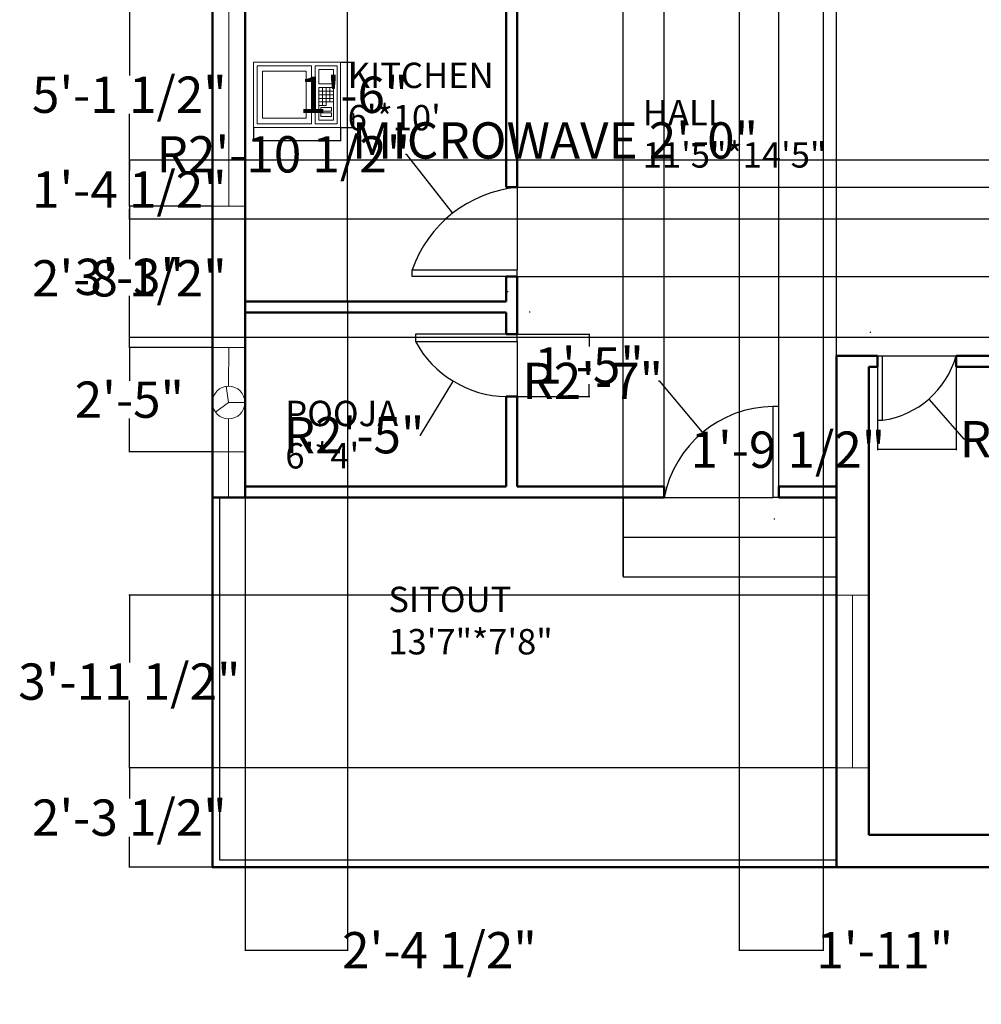
# Model space of a CAD drawing. Units: inches. Extents: x 430 to 924, y 262 to 758.
# Tile 1 of 3: x 430 to 695, y 262 to 534. Entities that reach past the tile are written whole.
import ezdxf

# ---------------------------------------------------------------- set-up
doc = ezdxf.new("R2010")
doc.units = ezdxf.units.IN
doc.header["$MEASUREMENT"] = 0
for name, color, linetype, lineweight in [('A-ANNO-DIMS', 2, 'Continuous', 18), ('A-AREA-IDEN', 7, 'Continuous', 25), ('A-DOOR', 4, 'Continuous', 25), ('A-EQPM', 8, 'Continuous', 18), ('A-FLOR', 7, 'Continuous', 25), ('A-FLOR-CASE', 9, 'Continuous', 25), ('A-FLOR-STRS', 7, 'Continuous', 25), ('A-GLAZ', 3, 'Continuous', 18), ('A-WALL', 7, 'Continuous', 50), ('M-HVAC-EQPM', 4, 'Continuous', 18)]:
    doc.layers.add(name, color=color, linetype=linetype, lineweight=lineweight)
doc.styles.get("Standard").update_dxf_attribs({"font": 'arial.ttf'})
doc.dimstyles.get("Standard").update_dxf_attribs({"dimtxt": 10, "dimasz": 0.18, "dimexe": 0.18, "dimexo": 0.0625, "dimgap": 0.09, "dimtad": 0, "dimtih": 1, "dimtoh": 1, "dimdec": 0, "dimzin": 0, "dimdsep": 46, "dimlunit": 3, "dimtxsty": 'Standard', "dimcen": 0.09, "dimadec": 0, "dimazin": 0, "dimtfac": 1, "dimtdec": 0, "dimtofl": 0, "dimtmove": 0, "dimatfit": 3, "dimfxl": 1, "dimtolj": 1, "dimtzin": 0, "dimarcsym": 0})

# ---------------------------------------------------------------- blocks, each defined once
blk = doc.blocks.new('Microwave')
for p, q in [((19, 7), (19, 11)), ((20, 11), (20, 7)), ((21, 7), (21, 11)), ((18, 10), (22, 10)), ((22, 9), (18, 9)), ((18, 8), (22, 8)), ((22, 7), (18, 7)), ((20, 6), (18, 6)), ((19, 6), (19, 7)), ((20, 7), (20, 6))]:
    blk.add_line(p, q)
for points in [[(0, 0), (0, 18), (24, 18), (24, 0)], [(1, 1), (1, 17), (16, 17), (16, 1)], [(17, 1), (17, 17), (23, 17), (23, 1)], [(2.5, 2.5), (2.5, 15.5), (14.5, 15.5), (14.5, 2.5)], [(18, 12), (18, 16), (22, 16), (22, 12)], [(18, 2), (18, 11), (22, 11), (22, 2)], [(18.5, 4.5), (18.5, 5.5), (21.5, 5.5), (21.5, 4.5)], [(18.5, 3), (18.5, 4), (21.5, 4), (21.5, 3)]]:
    blk.add_lwpolyline(points, close=True)
blk = doc.blocks.new('*D9')
at = {"layer": 'A-ANNO-DIMS', "color": 0, "lineweight": -2, "transparency": 16777216}
for p, q in [((494.67, 503.98), (494.67, 500.27)), ((518.67, 503.98), (518.67, 500.27)), ((494.85, 500.45), (518.49, 500.45)), ((518.67, 500.45), (518.85, 500.45))]:
    blk.add_line(p, q, dxfattribs=at)
at = {"layer": 'A-ANNO-DIMS', "color": 0, "transparency": 16777216}
for points in [[(494.85, 500.48), (494.85, 500.42), (494.67, 500.45)], [(518.49, 500.48), (518.49, 500.42), (518.67, 500.45)]]:
    blk.add_solid(points, dxfattribs=at)
at = {"layer": 'Defpoints', "color": 0, "transparency": 16777216}
for p in [(494.67, 504.05), (518.67, 504.05), (518.67, 500.45)]:
    blk.add_point(p, dxfattribs=at)
at = {"layer": 'A-ANNO-DIMS', "color": 0, "transparency": 16777216, "insert": (577.79, 500.45), "char_height": 10, "attachment_point": 5}
blk.add_mtext('\\A1;MICROWAVE 2\'-0"', dxfattribs=at)
blk = doc.blocks.new('*D10')
at = {"layer": 'A-ANNO-DIMS', "color": 0, "lineweight": -2, "transparency": 16777216}
for p, q in [((518.73, 522.05), (522.45, 522.05)), ((522.27, 521.87), (522.27, 518.24)), ((522.27, 504.23), (522.27, 507.85)), ((518.73, 504.05), (522.45, 504.05))]:
    blk.add_line(p, q, dxfattribs=at)
at = {"layer": 'A-ANNO-DIMS', "color": 0, "transparency": 16777216}
for points in [[(522.24, 521.87), (522.3, 521.87), (522.27, 522.05)], [(522.24, 504.23), (522.3, 504.23), (522.27, 504.05)]]:
    blk.add_solid(points, dxfattribs=at)
at = {"layer": 'Defpoints', "color": 0, "transparency": 16777216}
for p in [(518.67, 522.05), (522.27, 522.05), (518.67, 504.05)]:
    blk.add_point(p, dxfattribs=at)
at = {"layer": 'A-ANNO-DIMS', "color": 0, "transparency": 16777216, "insert": (522.27, 513.05), "char_height": 10, "attachment_point": 5}
blk.add_mtext('\\A1;1\'-6"', dxfattribs=at)
blk = doc.blocks.new('*D11')
at = {"layer": 'A-ANNO-DIMS', "color": 0, "lineweight": -2, "transparency": 16777216}
for p, q in [((523.75, 547.42), (523.75, 542.8)), ((553.75, 547.42), (553.75, 542.8)), ((523.93, 542.98), (553.57, 542.98)), ((553.75, 542.98), (553.93, 542.98))]:
    blk.add_line(p, q, dxfattribs=at)
at = {"layer": 'A-ANNO-DIMS', "color": 0, "transparency": 16777216}
for points in [[(523.93, 543.01), (523.93, 542.95), (523.75, 542.98)], [(553.57, 543.01), (553.57, 542.95), (553.75, 542.98)]]:
    blk.add_solid(points, dxfattribs=at)
at = {"layer": 'Defpoints', "color": 0, "transparency": 16777216}
for p in [(523.75, 547.48), (553.75, 547.48), (553.75, 542.98)]:
    blk.add_point(p, dxfattribs=at)
at = {"layer": 'A-ANNO-DIMS', "color": 0, "transparency": 16777216, "insert": (585.53, 542.98), "char_height": 10, "attachment_point": 5}
blk.add_mtext('\\A1;SINK 2\'-6"', dxfattribs=at)
blk = doc.blocks.new('*D28')
at = {"layer": 'A-ANNO-DIMS', "color": 0, "lineweight": -2, "transparency": 16777216}
for p, q in [((483.25, 543.78), (460.24, 543.78)), ((460.42, 543.6), (460.42, 518.31)), ((460.42, 482.49), (460.42, 507.78)), ((483.25, 482.31), (460.24, 482.31))]:
    blk.add_line(p, q, dxfattribs=at)
at = {"layer": 'A-ANNO-DIMS', "color": 0, "transparency": 16777216}
for points in [[(460.39, 543.6), (460.45, 543.6), (460.42, 543.78)], [(460.39, 482.49), (460.45, 482.49), (460.42, 482.31)]]:
    blk.add_solid(points, dxfattribs=at)
at = {"layer": 'Defpoints', "color": 0, "transparency": 16777216}
for p in [(483.32, 543.78), (460.42, 482.31), (483.32, 482.31)]:
    blk.add_point(p, dxfattribs=at)
at = {"layer": 'A-ANNO-DIMS', "color": 0, "transparency": 16777216, "insert": (460.42, 513.05), "char_height": 10, "attachment_point": 5}
blk.add_mtext('\\A1;5\'-1 1/2"', dxfattribs=at)
blk = doc.blocks.new('*D29')
at = {"layer": 'A-ANNO-DIMS', "color": 0, "lineweight": -2, "transparency": 16777216}
for p, q in [((483.25, 482.31), (460.24, 482.31)), ((460.42, 482.13), (460.42, 468.03)), ((460.42, 443.54), (460.42, 457.64)), ((483.25, 443.36), (460.24, 443.36))]:
    blk.add_line(p, q, dxfattribs=at)
at = {"layer": 'A-ANNO-DIMS', "color": 0, "transparency": 16777216}
for points in [[(460.39, 482.13), (460.45, 482.13), (460.42, 482.31)], [(460.39, 443.54), (460.45, 443.54), (460.42, 443.36)]]:
    blk.add_solid(points, dxfattribs=at)
at = {"layer": 'Defpoints', "color": 0, "transparency": 16777216}
for p in [(483.32, 482.31), (460.42, 443.36), (483.32, 443.36)]:
    blk.add_point(p, dxfattribs=at)
at = {"layer": 'A-ANNO-DIMS', "color": 0, "transparency": 16777216, "insert": (460.42, 462.84), "char_height": 10, "attachment_point": 5}
blk.add_mtext('\\A1;3\'-3"', dxfattribs=at)
blk = doc.blocks.new('*D30')
at = {"layer": 'A-ANNO-DIMS', "color": 0, "lineweight": -2, "transparency": 16777216}
for p, q in [((483.25, 443.36), (460.24, 443.36)), ((460.42, 443.18), (460.42, 434.17)), ((460.42, 414.78), (460.42, 423.78)), ((483.25, 414.6), (460.24, 414.6))]:
    blk.add_line(p, q, dxfattribs=at)
at = {"layer": 'A-ANNO-DIMS', "color": 0, "transparency": 16777216}
for points in [[(460.39, 443.18), (460.45, 443.18), (460.42, 443.36)], [(460.39, 414.78), (460.45, 414.78), (460.42, 414.6)]]:
    blk.add_solid(points, dxfattribs=at)
at = {"layer": 'Defpoints', "color": 0, "transparency": 16777216}
for p in [(483.32, 443.36), (460.42, 414.6), (483.32, 414.6)]:
    blk.add_point(p, dxfattribs=at)
at = {"layer": 'A-ANNO-DIMS', "color": 0, "transparency": 16777216, "insert": (460.42, 428.98), "char_height": 10, "attachment_point": 5}
blk.add_mtext('\\A1;2\'-5"', dxfattribs=at)
blk = doc.blocks.new('*D33')
at = {"layer": 'A-ANNO-DIMS', "color": 0, "lineweight": -2, "transparency": 16777216}
for p, q in [((655.25, 327.47), (460.24, 327.47)), ((460.42, 327.29), (460.42, 319.03)), ((460.42, 300.23), (460.42, 308.5)), ((655.25, 300.05), (460.24, 300.05))]:
    blk.add_line(p, q, dxfattribs=at)
at = {"layer": 'A-ANNO-DIMS', "color": 0, "transparency": 16777216}
for points in [[(460.39, 327.29), (460.45, 327.29), (460.42, 327.47)], [(460.39, 300.23), (460.45, 300.23), (460.42, 300.05)]]:
    blk.add_solid(points, dxfattribs=at)
at = {"layer": 'Defpoints', "color": 0, "transparency": 16777216}
for p in [(460.42, 327.47), (655.32, 327.47), (655.32, 300.05)]:
    blk.add_point(p, dxfattribs=at)
at = {"layer": 'A-ANNO-DIMS', "color": 0, "transparency": 16777216, "insert": (460.42, 313.76), "char_height": 10, "attachment_point": 5}
blk.add_mtext('\\A1;2\'-3 1/2"', dxfattribs=at)
blk = doc.blocks.new('*D34')
at = {"layer": 'A-ANNO-DIMS', "color": 0, "lineweight": -2, "transparency": 16777216}
for p, q in [((655.25, 375.05), (460.24, 375.05)), ((460.42, 374.87), (460.42, 356.53)), ((460.42, 327.65), (460.42, 346)), ((655.25, 327.47), (460.24, 327.47))]:
    blk.add_line(p, q, dxfattribs=at)
at = {"layer": 'A-ANNO-DIMS', "color": 0, "transparency": 16777216}
for points in [[(460.39, 374.87), (460.45, 374.87), (460.42, 375.05)], [(460.39, 327.65), (460.45, 327.65), (460.42, 327.47)]]:
    blk.add_solid(points, dxfattribs=at)
at = {"layer": 'Defpoints', "color": 0, "transparency": 16777216}
for p in [(460.42, 375.05), (655.32, 375.05), (655.32, 327.47)]:
    blk.add_point(p, dxfattribs=at)
at = {"layer": 'A-ANNO-DIMS', "color": 0, "transparency": 16777216, "insert": (460.42, 351.26), "char_height": 10, "attachment_point": 5}
blk.add_mtext('\\A1;3\'-11 1/2"', dxfattribs=at)
blk = doc.blocks.new('*D35')
at = {"layer": 'A-ANNO-DIMS', "color": 0, "lineweight": -2, "transparency": 16777216}
for p, q in [((596.53, 380.21), (596.53, 743.09)), ((596.71, 742.91), (608.45, 742.91)), ((655.14, 742.91), (643.39, 742.91)), ((655.32, 380.21), (655.32, 743.09))]:
    blk.add_line(p, q, dxfattribs=at)
at = {"layer": 'A-ANNO-DIMS', "color": 0, "transparency": 16777216}
for points in [[(596.71, 742.94), (596.71, 742.88), (596.53, 742.91)], [(655.14, 742.94), (655.14, 742.88), (655.32, 742.91)]]:
    blk.add_solid(points, dxfattribs=at)
at = {"layer": 'Defpoints', "color": 0, "transparency": 16777216}
for p in [(655.32, 742.91), (596.53, 380.15), (655.32, 380.15)]:
    blk.add_point(p, dxfattribs=at)
at = {"layer": 'A-ANNO-DIMS', "color": 0, "transparency": 16777216, "insert": (625.92, 742.91), "char_height": 10, "attachment_point": 5}
blk.add_mtext('\\A1;4\'-11"', dxfattribs=at)
blk = doc.blocks.new('*D39')
at = {"layer": 'A-ANNO-DIMS', "color": 0, "lineweight": -2, "transparency": 16777216}
for p, q in [((752.25, 478.73), (460.24, 478.73)), ((460.42, 478.55), (460.42, 467.71)), ((460.42, 446.34), (460.42, 457.18)), ((752.25, 446.16), (460.24, 446.16))]:
    blk.add_line(p, q, dxfattribs=at)
at = {"layer": 'A-ANNO-DIMS', "color": 0, "transparency": 16777216}
for points in [[(460.39, 478.55), (460.45, 478.55), (460.42, 478.73)], [(460.39, 446.34), (460.45, 446.34), (460.42, 446.16)]]:
    blk.add_solid(points, dxfattribs=at)
at = {"layer": 'Defpoints', "color": 0, "transparency": 16777216}
for p in [(460.42, 478.73), (752.32, 478.73), (752.32, 446.16)]:
    blk.add_point(p, dxfattribs=at)
at = {"layer": 'A-ANNO-DIMS', "color": 0, "transparency": 16777216, "insert": (460.42, 462.44), "char_height": 10, "attachment_point": 5}
blk.add_mtext('\\A1;2\'-8 1/2"', dxfattribs=at)
blk = doc.blocks.new('*D40')
at = {"layer": 'A-ANNO-DIMS', "color": 0, "lineweight": -2, "transparency": 16777216}
for p, q in [((752.25, 495.05), (460.24, 495.05)), ((460.42, 494.87), (460.42, 492.15)), ((460.42, 478.91), (460.42, 481.63)), ((752.25, 478.73), (460.24, 478.73))]:
    blk.add_line(p, q, dxfattribs=at)
at = {"layer": 'A-ANNO-DIMS', "color": 0, "transparency": 16777216}
for points in [[(460.39, 494.87), (460.45, 494.87), (460.42, 495.05)], [(460.39, 478.91), (460.45, 478.91), (460.42, 478.73)]]:
    blk.add_solid(points, dxfattribs=at)
at = {"layer": 'Defpoints', "color": 0, "transparency": 16777216}
for p in [(460.42, 495.05), (752.32, 495.05), (752.32, 478.73)]:
    blk.add_point(p, dxfattribs=at)
at = {"layer": 'A-ANNO-DIMS', "color": 0, "transparency": 16777216, "insert": (460.42, 486.89), "char_height": 10, "attachment_point": 5}
blk.add_mtext('\\A1;1\'-4 1/2"', dxfattribs=at)
blk = doc.blocks.new('*D42')
at = {"layer": 'A-ANNO-DIMS', "color": 0, "lineweight": -2, "transparency": 16777216}
for p, q in [((492.32, 455.99), (492.32, 277.02)), ((520.6, 455.99), (520.6, 277.02)), ((492.5, 277.2), (520.42, 277.2)), ((520.6, 277.2), (520.78, 277.2))]:
    blk.add_line(p, q, dxfattribs=at)
at = {"layer": 'A-ANNO-DIMS', "color": 0, "transparency": 16777216}
for points in [[(492.5, 277.23), (492.5, 277.17), (492.32, 277.2)], [(520.42, 277.23), (520.42, 277.17), (520.6, 277.2)]]:
    blk.add_solid(points, dxfattribs=at)
at = {"layer": 'Defpoints', "color": 0, "transparency": 16777216}
for p in [(492.32, 456.05), (520.6, 456.05), (520.6, 277.2)]:
    blk.add_point(p, dxfattribs=at)
at = {"layer": 'A-ANNO-DIMS', "color": 0, "transparency": 16777216, "insert": (545.9, 277.2), "char_height": 10, "attachment_point": 5}
blk.add_mtext('\\A1;2\'-4 1/2"', dxfattribs=at)
blk = doc.blocks.new('*D44')
at = {"layer": 'A-ANNO-DIMS', "color": 0, "lineweight": -2, "transparency": 16777216}
for p, q in [((567.38, 487.53), (854.35, 487.53)), ((854.17, 487.35), (854.17, 480.5)), ((854.17, 463.13), (854.17, 469.98)), ((567.38, 462.95), (854.35, 462.95))]:
    blk.add_line(p, q, dxfattribs=at)
at = {"layer": 'A-ANNO-DIMS', "color": 0, "transparency": 16777216}
for points in [[(854.14, 487.35), (854.2, 487.35), (854.17, 487.53)], [(854.14, 463.13), (854.2, 463.13), (854.17, 462.95)]]:
    blk.add_solid(points, dxfattribs=at)
at = {"layer": 'Defpoints', "color": 0, "transparency": 16777216}
for p in [(567.32, 487.53), (854.17, 487.53), (567.32, 462.95)]:
    blk.add_point(p, dxfattribs=at)
at = {"layer": 'A-ANNO-DIMS', "color": 0, "transparency": 16777216, "insert": (854.17, 475.24), "char_height": 10, "attachment_point": 5}
blk.add_mtext('\\A1;2\'-0 1/2"', dxfattribs=at)
blk = doc.blocks.new('*D46')
at = {"layer": 'A-ANNO-DIMS', "color": 0, "lineweight": -2, "transparency": 16777216}
for p, q in [((628.55, 575.99), (628.55, 277.02)), ((651.7, 575.99), (651.7, 277.02)), ((628.73, 277.2), (651.52, 277.2)), ((651.7, 277.2), (651.88, 277.2))]:
    blk.add_line(p, q, dxfattribs=at)
at = {"layer": 'A-ANNO-DIMS', "color": 0, "transparency": 16777216}
for points in [[(628.73, 277.23), (628.73, 277.17), (628.55, 277.2)], [(651.52, 277.23), (651.52, 277.17), (651.7, 277.2)]]:
    blk.add_solid(points, dxfattribs=at)
at = {"layer": 'Defpoints', "color": 0, "transparency": 16777216}
for p in [(628.55, 576.05), (651.7, 576.05), (651.7, 277.2)]:
    blk.add_point(p, dxfattribs=at)
at = {"layer": 'A-ANNO-DIMS', "color": 0, "transparency": 16777216, "insert": (668.68, 277.2), "char_height": 10, "attachment_point": 5}
blk.add_mtext('\\A1;1\'-11"', dxfattribs=at)
blk = doc.blocks.new('*D48')
at = {"layer": 'A-ANNO-DIMS', "color": 0, "lineweight": -2, "transparency": 16777216}
for p, q in [((607.88, 405.12), (607.88, 743.09)), ((608.06, 742.91), (639.32, 742.91)), ((639.5, 405.12), (639.5, 743.09)), ((639.5, 742.91), (639.68, 742.91))]:
    blk.add_line(p, q, dxfattribs=at)
at = {"layer": 'A-ANNO-DIMS', "color": 0, "transparency": 16777216}
for points in [[(608.06, 742.94), (608.06, 742.88), (607.88, 742.91)], [(639.32, 742.94), (639.32, 742.88), (639.5, 742.91)]]:
    blk.add_solid(points, dxfattribs=at)
at = {"layer": 'Defpoints', "color": 0, "transparency": 16777216}
for p in [(639.5, 742.91), (607.88, 405.05), (639.5, 405.05)]:
    blk.add_point(p, dxfattribs=at)
at = {"layer": 'A-ANNO-DIMS', "color": 0, "transparency": 16777216, "insert": (664.79, 742.91), "char_height": 10, "attachment_point": 5}
blk.add_mtext('\\A1;2\'-7 1/2"', dxfattribs=at)
blk = doc.blocks.new('*D49')
at = {"layer": 'A-ANNO-DIMS', "color": 0, "lineweight": -2, "transparency": 16777216}
for p, q in [((666.71, 437.99), (666.71, 415.02)), ((688.33, 437.99), (688.33, 415.02)), ((666.71, 415.2), (666.53, 415.2)), ((688.15, 415.2), (666.89, 415.2))]:
    blk.add_line(p, q, dxfattribs=at)
at = {"layer": 'A-ANNO-DIMS', "color": 0, "transparency": 16777216}
for points in [[(666.89, 415.23), (666.89, 415.17), (666.71, 415.2)], [(688.15, 415.23), (688.15, 415.17), (688.33, 415.2)]]:
    blk.add_solid(points, dxfattribs=at)
at = {"layer": 'Defpoints', "color": 0, "transparency": 16777216}
for p in [(666.71, 438.05), (688.33, 438.05), (666.71, 415.2)]:
    blk.add_point(p, dxfattribs=at)
at = {"layer": 'A-ANNO-DIMS', "color": 0, "transparency": 16777216, "insert": (641.97, 415.2), "char_height": 10, "attachment_point": 5}
blk.add_mtext('\\A1;1\'-9 1/2"', dxfattribs=at)
blk = doc.blocks.new('*D50')
at = {"layer": 'A-ANNO-DIMS', "color": 0, "lineweight": -2, "transparency": 16777216}
for p, q in [((564.38, 447.02), (587.35, 447.02)), ((587.17, 446.84), (587.17, 443.63)), ((587.17, 430.02), (587.17, 433.23)), ((564.38, 429.84), (587.35, 429.84))]:
    blk.add_line(p, q, dxfattribs=at)
at = {"layer": 'A-ANNO-DIMS', "color": 0, "transparency": 16777216}
for points in [[(587.14, 446.84), (587.2, 446.84), (587.17, 447.02)], [(587.14, 430.02), (587.2, 430.02), (587.17, 429.84)]]:
    blk.add_solid(points, dxfattribs=at)
at = {"layer": 'Defpoints', "color": 0, "transparency": 16777216}
for p in [(564.32, 447.02), (564.32, 429.84), (587.17, 429.84)]:
    blk.add_point(p, dxfattribs=at)
at = {"layer": 'A-ANNO-DIMS', "color": 0, "transparency": 16777216, "insert": (587.17, 438.43), "char_height": 10, "attachment_point": 5}
blk.add_mtext('\\A1;1\'-5"', dxfattribs=at)
blk = doc.blocks.new('*D54')
at = {"layer": 'A-ANNO-DIMS', "color": 0, "lineweight": -2, "transparency": 16777216}
for p, q in [((536.58, 496.62), (536.76, 496.62)), ((536.76, 496.62), (549.43, 480.49)), ((570.75, 453.23), (570.93, 453.23)), ((570.84, 453.14), (570.84, 453.32))]:
    blk.add_line(p, q, dxfattribs=at)
at = {"layer": 'A-ANNO-DIMS', "color": 0, "transparency": 16777216}
blk.add_solid([(549.45, 480.51), (549.4, 480.47), (549.54, 480.35)], dxfattribs=at)
at = {"layer": 'Defpoints', "color": 0, "transparency": 16777216}
for p in [(549.54, 480.35), (570.84, 453.23)]:
    blk.add_point(p, dxfattribs=at)
at = {"layer": 'A-ANNO-DIMS', "color": 0, "transparency": 16777216, "insert": (502.88, 496.62), "char_height": 10, "attachment_point": 5}
blk.add_mtext('\\A1;R2\'-10 1/2"', dxfattribs=at)
blk = doc.blocks.new('*D55')
at = {"layer": 'A-ANNO-DIMS', "color": 0, "lineweight": -2, "transparency": 16777216}
for p, q in [((564.69, 458.82), (564.87, 458.82)), ((564.78, 458.73), (564.78, 458.91)), ((540.71, 419.18), (549.64, 433.89)), ((540.53, 419.18), (540.71, 419.18))]:
    blk.add_line(p, q, dxfattribs=at)
at = {"layer": 'A-ANNO-DIMS', "color": 0, "transparency": 16777216}
blk.add_solid([(549.61, 433.91), (549.67, 433.87), (549.73, 434.04)], dxfattribs=at)
at = {"layer": 'Defpoints', "color": 0, "transparency": 16777216}
for p in [(564.78, 458.82), (549.73, 434.04)]:
    blk.add_point(p, dxfattribs=at)
at = {"layer": 'A-ANNO-DIMS', "color": 0, "transparency": 16777216, "insert": (522.36, 419.18), "char_height": 10, "attachment_point": 5}
blk.add_mtext('\\A1;R2\'-5"', dxfattribs=at)
blk = doc.blocks.new('*D56')
at = {"layer": 'A-ANNO-DIMS', "color": 0, "lineweight": -2, "transparency": 16777216}
for p, q in [((606.31, 434.15), (606.49, 434.15)), ((606.49, 434.15), (618.29, 420.04)), ((638.18, 396.15), (638.36, 396.15)), ((638.27, 396.06), (638.27, 396.24))]:
    blk.add_line(p, q, dxfattribs=at)
at = {"layer": 'A-ANNO-DIMS', "color": 0, "transparency": 16777216}
blk.add_solid([(618.32, 420.06), (618.27, 420.02), (618.41, 419.9)], dxfattribs=at)
at = {"layer": 'Defpoints', "color": 0, "transparency": 16777216}
for p in [(618.41, 419.9), (638.27, 396.15)]:
    blk.add_point(p, dxfattribs=at)
at = {"layer": 'A-ANNO-DIMS', "color": 0, "transparency": 16777216, "insert": (588.15, 434.15), "char_height": 10, "attachment_point": 5}
blk.add_mtext('\\A1;R2\'-7"', dxfattribs=at)
blk = doc.blocks.new('*D57')
at = {"layer": 'A-ANNO-DIMS', "color": 0, "lineweight": -2, "transparency": 16777216}
for p, q in [((664.61, 447.63), (664.79, 447.63)), ((664.7, 447.54), (664.7, 447.72)), ((690.53, 418.08), (680.96, 429.02)), ((690.71, 418.08), (690.53, 418.08))]:
    blk.add_line(p, q, dxfattribs=at)
at = {"layer": 'A-ANNO-DIMS', "color": 0, "transparency": 16777216}
blk.add_solid([(680.98, 429.04), (680.94, 429), (680.84, 429.16)], dxfattribs=at)
at = {"layer": 'Defpoints', "color": 0, "transparency": 16777216}
for p in [(664.7, 447.63), (680.84, 429.16)]:
    blk.add_point(p, dxfattribs=at)
at = {"layer": 'A-ANNO-DIMS', "color": 0, "transparency": 16777216, "insert": (720.53, 418.08), "char_height": 10, "attachment_point": 5}
blk.add_mtext('\\A1;R2\'-0 1/2"', dxfattribs=at)

msp = doc.modelspace()

# ---------------------------------------------------------------- linework, layer by layer
at = {"layer": 'A-DOOR'}
for p, q in [((567.32, 487.53), (567.32, 464.78)), ((538.34, 462.95), (538.34, 464.78)), ((538.34, 464.78), (567.32, 464.78)), ((567.32, 462.95), (567.32, 464.78)), ((564.32, 462.95), (538.34, 462.95)), ((567.32, 447.02), (539.28, 447.02)), ((539.28, 447.02), (539.28, 445.04)), ((567.32, 445.04), (567.32, 447.02)), ((539.28, 445.04), (567.32, 445.04)), ((567.32, 445.04), (567.32, 429.84)), ((666.71, 441.05), (688.33, 441.05)), ((668.05, 423.33), (668.05, 441.05)), ((666.71, 438.05), (666.71, 423.33)), ((639.5, 427.11), (637.84, 427.11)), ((637.84, 427.11), (637.84, 402.14)), ((639.5, 405.05), (639.5, 427.11)), ((666.71, 423.33), (668.05, 423.33)), ((607.88, 402.05), (637.84, 402.05)), ((637.84, 402.14), (639.5, 402.14))]:
    msp.add_line(p, q, dxfattribs=at)
for centre, radius, start, end in [((570.84, 453.23), 34.49, 95.8576, 160.4254), ((564.78, 458.82), 28.98, 208.3786, 269.0869), ((664.7, 447.63), 24.53, 277.8641, 344.4616), ((638.27, 396.15), 30.96, 90.8013, 169.0102)]:
    msp.add_arc(centre, radius, start, end, dxfattribs=at)
at = {"layer": 'A-FLOR'}
msp.add_lwpolyline([(655.32, 302.05), (485.32, 302.05), (485.32, 402.05)], dxfattribs=at)
at = {"layer": 'A-FLOR-CASE'}
msp.add_line((520.6, 456.05), (520.6, 541.01), dxfattribs=at)
at = {"layer": 'A-FLOR-STRS'}
for p, q in [((596.53, 402.05), (596.53, 380.15)), ((596.53, 391.1), (655.32, 391.1)), ((596.53, 380.15), (655.32, 380.15))]:
    msp.add_line(p, q, dxfattribs=at)
at = {"layer": 'A-GLAZ'}
for p, q in [((487.82, 543.78), (487.82, 482.31)), ((483.32, 482.31), (492.32, 482.31)), ((487.82, 443.36), (487.77, 432.71)), ((487.77, 423.71), (487.77, 402.05)), ((483.32, 414.6), (492.32, 414.6)), ((655.32, 375.05), (664.32, 375.05)), ((659.82, 375.05), (659.82, 327.47)), ((655.32, 327.47), (664.32, 327.47))]:
    msp.add_line(p, q, dxfattribs=at)
msp.add_lwpolyline([(483.32, 443.36), (492.32, 443.36)], dxfattribs=at)
at = {"layer": 'A-WALL'}
for p, q in [((492.32, 402.05), (492.32, 576.05)), ((564.32, 498.05), (564.32, 576.05)), ((567.32, 498.05), (567.32, 576.05)), ((564.32, 498.05), (564.32, 487.53)), ((567.32, 487.53), (567.32, 498.05)), ((564.32, 487.53), (567.32, 487.53)), ((564.32, 462.95), (567.32, 462.95)), ((564.32, 456.05), (564.32, 462.95)), ((567.32, 447.02), (567.32, 462.95)), ((492.32, 456.05), (564.32, 456.05)), ((492.32, 453.05), (564.32, 453.05)), ((564.32, 447.02), (564.32, 453.05)), ((564.32, 447.02), (567.32, 447.02)), ((655.32, 309.05), (655.32, 441.05)), ((664.32, 441.05), (655.32, 441.05)), ((666.71, 441.05), (664.32, 441.05)), ((666.71, 441.05), (666.71, 438.05)), ((706.32, 441.05), (688.33, 441.05)), ((688.33, 441.05), (688.33, 438.05)), ((664.32, 309.05), (664.32, 438.05)), ((666.71, 438.05), (664.32, 438.05)), ((703.32, 438.05), (688.33, 438.05)), ((564.32, 405.05), (564.32, 429.84)), ((564.32, 429.84), (567.32, 429.84)), ((567.32, 405.05), (567.32, 429.84)), ((492.32, 405.05), (564.32, 405.05)), ((567.32, 405.05), (607.88, 405.05)), ((607.88, 405.05), (607.88, 402.05)), ((655.32, 405.05), (639.5, 405.05)), ((639.5, 405.05), (639.5, 402.05)), ((655.32, 405.05), (655.32, 405.05)), ((492.32, 402.05), (483.32, 402.05)), ((492.32, 402.05), (607.88, 402.05)), ((639.5, 402.05), (655.32, 402.05)), ((655.32, 309.05), (655.32, 300.05)), ((822.32, 309.05), (664.32, 309.05))]:
    msp.add_line(p, q, dxfattribs=at)
msp.add_lwpolyline([(831.32, 720.05), (831.32, 300.05), (483.32, 300.05), (483.32, 720.05)], close=True, dxfattribs=at)
at = {"layer": 'M-HVAC-EQPM'}
for q in [(487.11, 432.66), (484.13, 425.57), (492.27, 428.21)]:
    msp.add_line((487.77, 428.21), q, dxfattribs=at)
msp.add_circle((487.77, 428.21), 4.5, dxfattribs=at)

# ---------------------------------------------------------------- block references
at = {"layer": 'A-EQPM'}
msp.add_blockref('Microwave', (494.67, 504.05), dxfattribs=at)

# ---------------------------------------------------------------- texts
at = {"layer": 'A-AREA-IDEN', "char_height": 7, "attachment_point": 1}
for s, insert in [("KITCHEN\\P6'*10'", (520.6, 521.89)), ('HALL\\P11\'5"*14\'5"', (601.94, 511.63)), ("POOJA\\P6'*4'", (503.41, 428.68)), ('SITOUT\\P13\'7"*7\'8"', (531.81, 377.42))]:
    msp.add_mtext_dynamic_manual_height_columns(s, width=58.4467, gutter_width=1, heights=[0], dxfattribs=dict(at, insert=insert))

# ---------------------------------------------------------------- dimensions: what is measured, and where the dimension line sits
at = {"layer": 'A-ANNO-DIMS'}
for base, p1, p2, picture, middle in [((639.5, 742.91), (607.88, 405.05), (639.5, 405.05), '*D48', (664.79, 742.91)), ((655.32, 742.91), (596.53, 380.15), (655.32, 380.15), '*D35', (625.92, 742.91)), ((651.7007, 277.1992), (628.5501, 576.0542), (651.7007, 576.0542), '*D46', (668.6761, 277.1992)), ((520.6, 277.2), (492.32, 456.05), (520.6, 456.05), '*D42', (545.9, 277.2))]:
    dim = msp.add_linear_dim(base=base, p1=p1, p2=p2, dimstyle='Standard', override={"dimdec": 1, "dimlfac": 1, "dimrnd": 0, "dimzin": 1, "dimdsep": 46, "dimlunit": 4, "dimfrac": 2}, dxfattribs=at)
    dim.commit()
    dim.dimension.update_dxf_attribs({"geometry": picture, "text_midpoint": middle})
for base, p1, p2, text, picture, middle in [((553.75, 542.98), (523.75, 547.48), (553.75, 547.48), 'SINK <>', '*D11', (585.53, 542.98)), ((518.67, 500.45), (494.67, 504.05), (518.67, 504.05), 'MICROWAVE <>', '*D9', (577.79, 500.45))]:
    dim = msp.add_linear_dim(base=base, p1=p1, p2=p2, text=text, dimstyle='Standard', override={"dimdec": 1, "dimlfac": 1, "dimrnd": 0, "dimzin": 1, "dimdsep": 46, "dimlunit": 4, "dimfrac": 2}, dxfattribs=at)
    dim.commit()
    dim.dimension.update_dxf_attribs({"geometry": picture, "text_midpoint": middle})
for base, p1, p2, angle, picture, middle in [((460.42, 482.31), (483.32, 543.78), (483.32, 482.31), 90, '*D28', (460.42, 513.05)), ((522.27, 522.05), (518.67, 504.05), (518.67, 522.05), 90, '*D10', (522.27, 513.05)), ((460.42, 495.05), (752.32, 478.73), (752.32, 495.05), 90, '*D40', (460.42, 486.89)), ((854.17, 487.53), (567.32, 462.95), (567.32, 487.53), 90, '*D44', (854.17, 475.24)), ((460.4199, 443.3563), (483.3156, 482.3144), (483.3156, 443.3563), 90, '*D29', (460.4199, 462.8354)), ((460.42, 478.73), (752.32, 446.16), (752.32, 478.73), 90, '*D39', (460.42, 462.44)), ((587.17, 429.84), (564.32, 447.02), (564.32, 429.84), 270, '*D50', (587.17, 438.43)), ((460.42, 414.6), (483.32, 443.36), (483.32, 414.6), 90, '*D30', (460.42, 428.98)), ((666.71, 415.2), (688.33, 438.05), (666.71, 438.05), 180, '*D49', (641.97, 415.2)), ((460.42, 375.05), (655.32, 327.47), (655.32, 375.05), 90, '*D34', (460.42, 351.26)), ((460.42, 327.47), (655.32, 300.05), (655.32, 327.47), 90, '*D33', (460.42, 313.76))]:
    dim = msp.add_linear_dim(base=base, p1=p1, p2=p2, angle=angle, dimstyle='Standard', override={"dimdec": 1, "dimlfac": 1, "dimrnd": 0, "dimzin": 1, "dimdsep": 46, "dimlunit": 4, "dimfrac": 2}, dxfattribs=at)
    dim.commit()
    dim.dimension.update_dxf_attribs({"geometry": picture, "text_midpoint": middle})
for center, mpoint, picture, middle in [((570.84, 453.23), (549.54, 480.35), '*D54', (502.88, 496.62)), ((564.78, 458.82), (549.73, 434.04), '*D55', (522.36, 419.18)), ((664.7, 447.63), (680.84, 429.16), '*D57', (720.53, 418.08)), ((638.27, 396.15), (618.41, 419.9), '*D56', (588.15, 434.15))]:
    dim = msp.add_radius_dim(center=center, mpoint=mpoint, dimstyle='Standard', override={"dimdec": 1, "dimlfac": 1, "dimrnd": 0, "dimzin": 1, "dimdsep": 46, "dimlunit": 4, "dimfrac": 2}, dxfattribs=at)
    dim.commit()
    dim.dimension.update_dxf_attribs({"geometry": picture, "text_midpoint": middle, "dimtype": 164})

doc.saveas('drawing.dxf')
